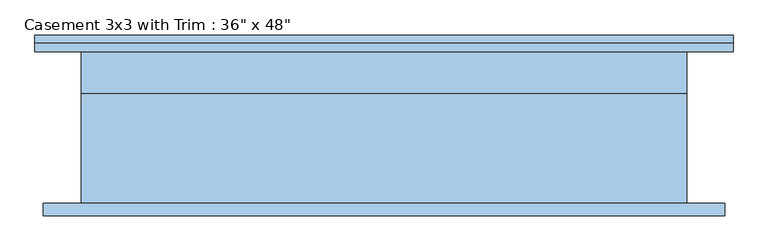
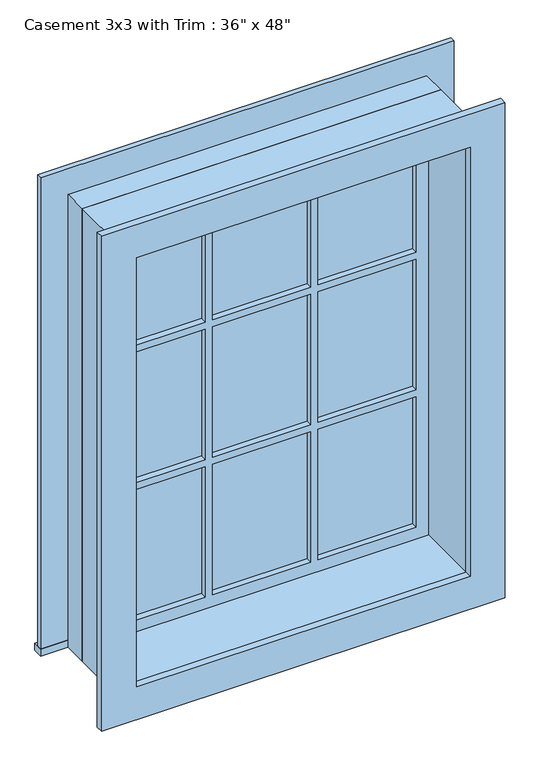
"""IFC4 building model written with IfcOpenShell, lengths in millimetres: window geometry."""

from ifc_helpers import new_model, si_unit, frame, origin, place, context, project, spatial, polyline, outline, extrude, source, transform, mapped, element, save


def window_642cfea4(model_context):
    return source(origin(), model_context, "Body", "SweptSolid", [
        extrude(outline(polyline([(-527.05, 139.7), (527.05, 139.7), (527.05, 114.3), (-527.05, 114.3), (-527.05, 139.7)])), frame((0.0, 0.0, 609.6), z_axis=(0.0, 0.0, 1.0), x_axis=(1.0, 0.0, 0.0)), (0.0, 0.0, 1.0), 19.05),
        extrude(outline(polyline([(1809.75, -438.15), (1809.75, 438.15), (628.65, 438.15), (628.65, 527.05), (1898.65, 527.05), (1898.65, -527.05), (628.65, -527.05), (628.65, -438.15), (1809.75, -438.15)])), frame((0.0, 114.3, 0.0), z_axis=(0.0, 1.0, 0.0), x_axis=(0.0, 0.0, 1.0)), (0.0, 0.0, 1.0), 12.7),
        extrude(outline(polyline([(143.9333333, 79.375), (393.7, 79.375), (393.7, 66.675), (143.9333333, 66.675), (143.9333333, 79.375)])), frame((0.0, 0.0, 1413.9333333), z_axis=(0.0, 0.0, 1.0), x_axis=(1.0, 0.0, 0.0)), (0.0, 0.0, 1.0), 351.3666667),
        extrude(outline(polyline([(-124.8833333, 79.375), (124.8833333, 79.375), (124.8833333, 66.675), (-124.8833333, 66.675), (-124.8833333, 79.375)])), frame((0.0, 0.0, 1413.9333333), z_axis=(0.0, 0.0, 1.0), x_axis=(1.0, 0.0, 0.0)), (0.0, 0.0, 1.0), 351.3666667),
        extrude(outline(polyline([(-393.7, 79.375), (-143.9333333, 79.375), (-143.9333333, 66.675), (-393.7, 66.675), (-393.7, 79.375)])), frame((0.0, 0.0, 1413.9333333), z_axis=(0.0, 0.0, 1.0), x_axis=(1.0, 0.0, 0.0)), (0.0, 0.0, 1.0), 351.3666667),
        extrude(outline(polyline([(-393.7, 79.375), (-143.9333333, 79.375), (-143.9333333, 66.675), (-393.7, 66.675), (-393.7, 79.375)])), frame((0.0, 0.0, 1043.5166667), z_axis=(0.0, 0.0, 1.0), x_axis=(1.0, 0.0, 0.0)), (0.0, 0.0, 1.0), 351.3666667),
        extrude(outline(polyline([(-124.8833333, 79.375), (124.8833333, 79.375), (124.8833333, 66.675), (-124.8833333, 66.675), (-124.8833333, 79.375)])), frame((0.0, 0.0, 1043.5166667), z_axis=(0.0, 0.0, 1.0), x_axis=(1.0, 0.0, 0.0)), (0.0, 0.0, 1.0), 351.3666667),
        extrude(outline(polyline([(143.9333333, 79.375), (393.7, 79.375), (393.7, 66.675), (143.9333333, 66.675), (143.9333333, 79.375)])), frame((0.0, 0.0, 1043.5166667), z_axis=(0.0, 0.0, 1.0), x_axis=(1.0, 0.0, 0.0)), (0.0, 0.0, 1.0), 351.3666667),
        extrude(outline(polyline([(143.9333333, 79.375), (393.7, 79.375), (393.7, 66.675), (143.9333333, 66.675), (143.9333333, 79.375)])), frame((0.0, 0.0, 673.1), z_axis=(0.0, 0.0, 1.0), x_axis=(1.0, 0.0, 0.0)), (0.0, 0.0, 1.0), 351.3666667),
        extrude(outline(polyline([(-124.8833333, 79.375), (124.8833333, 79.375), (124.8833333, 66.675), (-124.8833333, 66.675), (-124.8833333, 79.375)])), frame((0.0, 0.0, 673.1), z_axis=(0.0, 0.0, 1.0), x_axis=(1.0, 0.0, 0.0)), (0.0, 0.0, 1.0), 351.3666667),
        extrude(outline(polyline([(-393.7, 79.375), (-143.9333333, 79.375), (-143.9333333, 66.675), (-393.7, 66.675), (-393.7, 79.375)])), frame((0.0, 0.0, 673.1), z_axis=(0.0, 0.0, 1.0), x_axis=(1.0, 0.0, 0.0)), (0.0, 0.0, 1.0), 351.3666667),
        extrude(outline(polyline([(1885.95, 514.35), (1885.95, -514.35), (552.45, -514.35), (552.45, 514.35), (1885.95, 514.35)]), holes=[polyline([(1797.05, 425.45), (641.35, 425.45), (641.35, -425.45), (1797.05, -425.45), (1797.05, 425.45)])]), frame((0.0, -133.35, 0.0), z_axis=(0.0, 1.0, 0.0), x_axis=(0.0, 0.0, 1.0)), (0.0, 0.0, 1.0), 19.05),
        extrude(outline(polyline([(1809.75, -438.15), (628.65, -438.15), (628.65, 438.15), (1809.75, 438.15), (1809.75, -438.15)]), holes=[polyline([(1765.3, -143.9333333), (1413.9333333, -143.9333333), (1413.9333333, -393.7), (1765.3, -393.7), (1765.3, -143.9333333)]), polyline([(1394.8833333, -143.9333333), (1043.5166667, -143.9333333), (1043.5166667, -393.7), (1394.8833333, -393.7), (1394.8833333, -143.9333333)]), polyline([(1024.4666667, -143.9333333), (673.1, -143.9333333), (673.1, -393.7), (1024.4666667, -393.7), (1024.4666667, -143.9333333)]), polyline([(1765.3, 124.8833333), (1413.9333333, 124.8833333), (1413.9333333, -124.8833333), (1765.3, -124.8833333), (1765.3, 124.8833333)]), polyline([(1394.8833333, 124.8833333), (1043.5166667, 124.8833333), (1043.5166667, -124.8833333), (1394.8833333, -124.8833333), (1394.8833333, 124.8833333)]), polyline([(1024.4666667, 124.8833333), (673.1, 124.8833333), (673.1, -124.8833333), (1024.4666667, -124.8833333), (1024.4666667, 124.8833333)]), polyline([(1765.3, 393.7), (1413.9333333, 393.7), (1413.9333333, 143.9333333), (1765.3, 143.9333333), (1765.3, 393.7)]), polyline([(1394.8833333, 393.7), (1043.5166667, 393.7), (1043.5166667, 143.9333333), (1394.8833333, 143.9333333), (1394.8833333, 393.7)]), polyline([(1024.4666667, 393.7), (673.1, 393.7), (673.1, 143.9333333), (1024.4666667, 143.9333333), (1024.4666667, 393.7)])]), frame((0.0, 50.8, 0.0), z_axis=(0.0, 1.0, 0.0), x_axis=(0.0, 0.0, 1.0)), (0.0, 0.0, 1.0), 44.45),
        extrude(outline(polyline([(1828.8, -457.2), (609.6, -457.2), (609.6, 457.2), (1828.8, 457.2), (1828.8, -457.2)]), holes=[polyline([(1797.05, -425.45), (1797.05, 425.45), (641.35, 425.45), (641.35, -425.45), (1797.05, -425.45)])]), frame((0.0, -114.3, 0.0), z_axis=(0.0, 1.0, 0.0), x_axis=(0.0, 0.0, 1.0)), (0.0, 0.0, 1.0), 165.1),
        extrude(outline(polyline([(1828.8, 457.2), (1828.8, -457.2), (609.6, -457.2), (609.6, 457.2), (1828.8, 457.2)]), holes=[polyline([(1809.75, 438.15), (628.65, 438.15), (628.65, -438.15), (1809.75, -438.15), (1809.75, 438.15)])]), frame((0.0, 50.8, 0.0), z_axis=(0.0, 1.0, 0.0), x_axis=(0.0, 0.0, 1.0)), (0.0, 0.0, 1.0), 63.5),
    ])


if __name__ == "__main__":
    model = new_model("IFC4")
    model_context = context("Model", 3, world=origin())
    ifc_project = project(units=[si_unit("LENGTHUNIT", "METRE", prefix="MILLI")], contexts=[model_context])
    site = spatial("IfcSite", under=ifc_project)
    building = spatial("IfcBuilding", under=site)
    placement = place(None, origin())
    window_shape = window_642cfea4(model_context)
    element("IfcWindow", 1, ObjectType="Casement 3x3 with Trim : 36\" x 48\"", at=placement, inside=building, context=model_context, shape_type="MappedRepresentation", body=[
        mapped(window_shape, transform((0.0, 0.0, 0.0), x_axis=(1.0, 0.0, 0.0), y_axis=(0.0, 1.0, 0.0), z_axis=(0.0, 0.0, 1.0))),
    ])
    save(model, "model.ifc")

# Revit data of these elements
# Type "Casement 3x3 with Trim : 36\" x 48\""
#   Type Mark = "11"
#   Construction Type Id = "GSP4R"
#   Assembly Code = "B2020100"
#   Analytic Construction = "1/8 in Pilkington single glazing"
#   Visual Light Transmittance = 0.9
#   Solar Heat Gain Coefficient = 0.78
#   Heat Transfer Coefficient (U) = 0.6496 BTU/(h·ft²·°F)
#   Height = 4' - 0"
#   Default Sill Height = 2' - 0"
#   Trim Projection - Ext. = 0' - 0 1/2"
#   Trim Projection - Int. = 0' - 0 3/4"
#   Trim Width - Exterior = 0' - 3 1/2"
#   Trim Width - Interior = 0' - 3 1/2"
#   Width = 3' - 0"
#   Window Inset = 0' - 0 3/4"
#   Define Thermal Properties by = 1
#   Glass Pane Material = Glass
#   Sash Material = Softwood, Lumber
#   Trim Exterior Material = Trim
#   Trim Interior Material = Trim
#   Wall Closure = (empty or 0)
# Element 1 (IfcWindow, "Casement 3x3 with Trim : 36\" x 48\"")
#   Materials on its faces: "Softwood, Lumber", "Glass", "Trim"
# Materials
#   "Glass": class "Glass", colour RGB 0 128 192, transparency 0.75, Description = "Soda Lime Glass", Cost = 0
#   "Softwood, Lumber": class "Wood", colour RGB 223 192 134, transparency 0, Description = "Pinus Echinata", Cost = 0
#   "Trim": class "Wood", colour RGB 224 178 126, transparency 0
